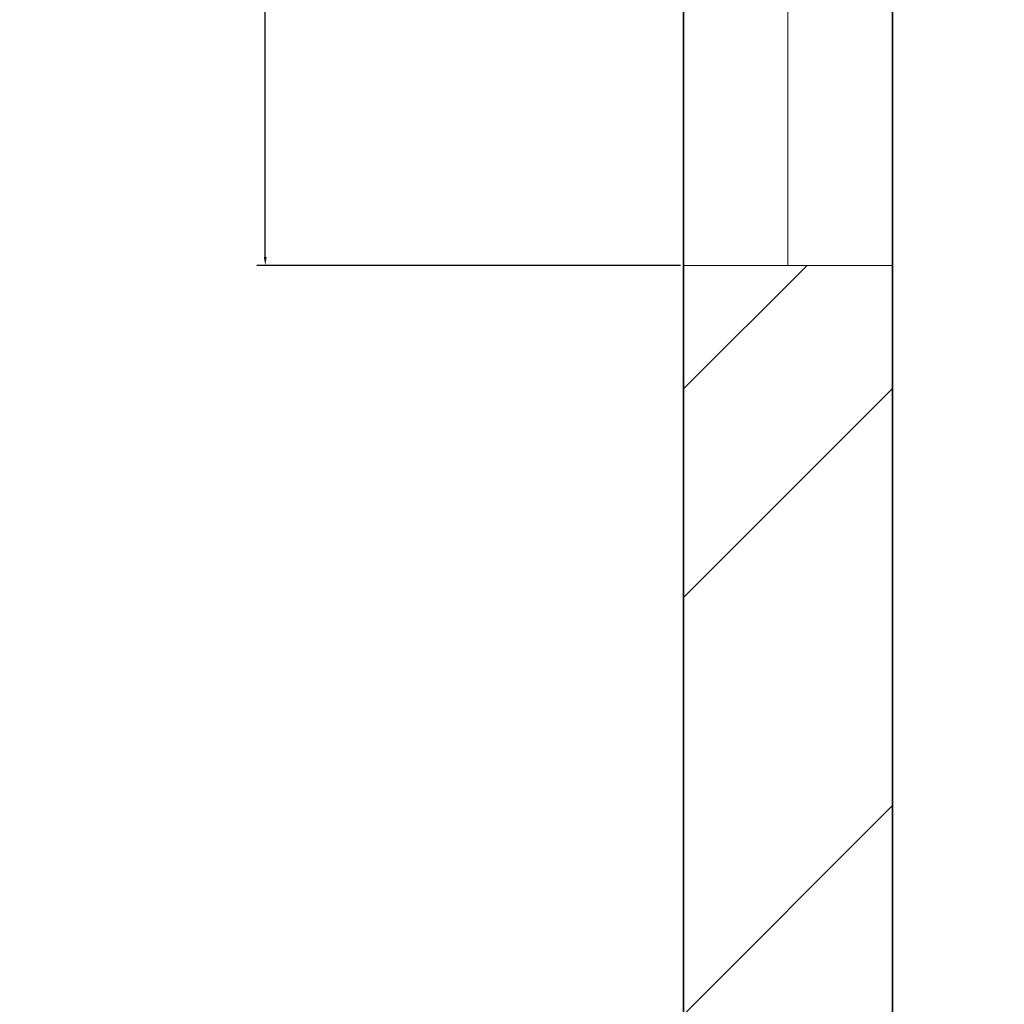
# Model space of a CAD drawing. Units: inches. Extents: x 1962 to 2771, y 1245 to 2660.
# Tile 23 of 114: x 2072 to 2093, y 1831 to 1852. Entities that reach past the tile are written whole.
import ezdxf

# ---------------------------------------------------------------- set-up
doc = ezdxf.new("R2010")
doc.units = ezdxf.units.IN
for name, color, linetype, lineweight in [('A-ANNO-DIMS', 2, 'Continuous', 18), ('A-GLAZ', 4, 'Continuous', 18), ('A-WALL', 7, 'Continuous', 35), ('A-WALL-PATT', 252, 'Continuous', 13)]:
    doc.layers.add(name, color=color, linetype=linetype, lineweight=lineweight)
doc.styles.get("Standard").update_dxf_attribs({"font": 'arial.ttf'})
doc.dimstyles.get("Standard").update_dxf_attribs({"dimtxt": 0.18, "dimasz": 0.18, "dimexe": 0.18, "dimexo": 0.0625, "dimgap": 0.09, "dimtad": 0, "dimtih": 1, "dimtoh": 1, "dimdec": 4, "dimzin": 0, "dimdsep": 46, "dimtxsty": 'Standard', "dimcen": 0.09, "dimadec": 0, "dimazin": 0, "dimtfac": 1, "dimtdec": 4, "dimtofl": 0, "dimtmove": 0, "dimatfit": 3, "dimfxl": 1, "dimtolj": 1, "dimtzin": 0, "dimarcsym": 0})

# ---------------------------------------------------------------- blocks, each defined once
blk = doc.blocks.new('WIN-60IN-A')
for p, q in [((2.25, 60), (2.25, 0)), ((2.25, 0), (0, 0)), ((0, 0), (4.5, 0))]:
    blk.add_line(p, q)
blk = doc.blocks.new('*D22')
at = {"layer": 'A-ANNO-DIMS', "color": 0, "lineweight": -2, "transparency": 16777216}
for p, q in [((2086.245, 1906.501), (2077.127, 1906.501)), ((2077.307, 1906.321), (2077.307, 1876.683)), ((2077.307, 1846.681), (2077.307, 1876.319)), ((2086.245, 1846.501), (2077.127, 1846.501))]:
    blk.add_line(p, q, dxfattribs=at)
at = {"layer": 'A-ANNO-DIMS', "color": 0, "transparency": 16777216}
for points in [[(2077.277, 1906.321), (2077.337, 1906.321), (2077.307, 1906.501)], [(2077.277, 1846.681), (2077.337, 1846.681), (2077.307, 1846.501)]]:
    blk.add_solid(points, dxfattribs=at)
at = {"layer": 'Defpoints', "color": 0, "transparency": 16777216}
for p in [(2077.307, 1906.501), (2086.307, 1906.501), (2086.307, 1846.501)]:
    blk.add_point(p, dxfattribs=at)
at = {"layer": 'A-ANNO-DIMS', "color": 0, "transparency": 16777216, "insert": (2077.307, 1876.501), "char_height": 0.18, "attachment_point": 5}
blk.add_mtext('\\A1;W3A 60 TYP.', dxfattribs=at)

msp = doc.modelspace()

# ---------------------------------------------------------------- hatches: boundary and pattern name
at = {"layer": 'A-WALL-PATT'}
h = msp.add_hatch(dxfattribs=at)
h.set_pattern_fill('ANSI32', color=256)
h.paths.add_polyline_path([(2090.8074, 2467.3437), (2141.6481, 2467.3437), (2141.6481, 2469.5937), (2141.6481, 2471.8437), (2086.3074, 2471.8437), (2086.3074, 2422.5333), (2090.8074, 2422.5333)])
h.paths.add_polyline_path([(2282.7664, 2471.8437), (2204.8982, 2471.8437), (2204.8982, 2467.3437), (2234.8074, 2467.3437), (2234.8074, 2311.3437), (2228.7492, 2311.3437), (2228.7492, 2306.8437), (2234.8074, 2306.8437), (2331.9227, 2306.8437), (2331.9227, 2309.0937), (2331.9227, 2311.3437), (2239.3074, 2311.3437), (2239.3074, 2467.3437), (2282.7664, 2467.3437), (2282.7664, 2469.5937)])
h.paths.add_polyline_path([(2471.4531, 2519.8437), (2552.011, 2519.8437), (2564.3996, 2519.8437), (2564.3996, 2511.1389), (2568.8996, 2511.1389), (2568.8996, 2524.3437), (2466.9531, 2524.3437), (2466.9531, 2471.8437), (2450.0749, 2471.8437), (2446.4672, 2471.8437), (2446.4672, 2467.3437), (2450.0749, 2467.3437), (2475.9988, 2467.3437), (2475.9988, 2469.5937), (2475.9988, 2471.8437), (2471.4531, 2471.8437)])
h.paths.add_polyline_path([(2575.2231, 2469.5937), (2575.2231, 2471.8437), (2568.8996, 2471.8437), (2568.8996, 2487.1389), (2564.3996, 2487.1389), (2564.3996, 2471.8437), (2556.511, 2471.8437), (2499.2904, 2471.8437), (2499.2904, 2467.3437), (2507.8074, 2467.3437), (2507.8074, 2311.3437), (2414.863, 2311.3437), (2414.863, 2306.8437), (2512.3074, 2306.8437), (2517.0114, 2306.8437), (2517.0114, 2309.0937), (2517.0114, 2311.3437), (2512.3074, 2311.3437), (2512.3074, 2467.3437), (2575.2231, 2467.3437)])
h.paths.add_polyline_path([(2660.8074, 2471.8437), (2600.9602, 2471.8437), (2600.9602, 2467.3437), (2656.3074, 2467.3437), (2656.3074, 2432.5704), (2660.8074, 2432.5704)])
h.paths.add_polyline_path([(2660.8074, 2372.5704), (2656.3074, 2372.5704), (2656.3074, 2311.3437), (2600.276, 2311.3437), (2600.276, 2309.0937), (2600.276, 2306.8437), (2656.3074, 2306.8437), (2656.3074, 2296.2593), (2660.8074, 2296.2593)])
h.paths.add_polyline_path([(2572.3074, 2306.8437), (2577.1385, 2306.8437), (2577.1385, 2311.3437), (2551.082, 2311.3437), (2551.082, 2306.8437), (2567.8074, 2306.8437), (2567.8074, 2258.8437), (2540.0574, 2258.8437), (2540.0574, 2256.5937), (2540.0574, 2254.3437), (2567.8074, 2254.3437), (2656.3074, 2254.3437), (2656.3074, 2236.9085), (2660.8074, 2236.9085), (2660.8074, 2272.2593), (2656.3074, 2272.2593), (2656.3074, 2258.8437), (2572.3074, 2258.8437)])
h.paths.add_polyline_path([(2512.3074, 2254.3437), (2518.8716, 2254.3437), (2518.8716, 2256.5937), (2518.8716, 2258.8437), (2507.8074, 2258.8437), (2507.8074, 2177.8437), (2567.8074, 2177.8437), (2567.8074, 2172.9628), (2572.3074, 2172.9628), (2572.3074, 2177.8437), (2656.3074, 2177.8437), (2656.3074, 2166.4846), (2660.8074, 2166.4846), (2660.8074, 2200.9085), (2656.3074, 2200.9085), (2656.3074, 2182.3437), (2512.3074, 2182.3437)])
h.paths.add_polyline_path([(2656.3074, 2129.8437), (2572.3074, 2129.8437), (2572.3074, 2150.3044), (2570.0574, 2150.3044), (2567.8074, 2150.3044), (2567.8074, 2129.8437), (2507.8074, 2129.8437), (2507.8074, 2116.3027), (2510.0574, 2116.3027), (2512.3074, 2116.3027), (2512.3074, 2125.3437), (2567.8074, 2125.3437), (2572.3074, 2125.3437), (2656.3074, 2125.3437)])
h.paths.add_polyline_path([(2090.8074, 2362.5333), (2086.3074, 2362.5333), (2086.3074, 2298.6242), (2090.8074, 2298.6242), (2090.8074, 2306.8437), (2174.8074, 2306.8437), (2174.8074, 2286.4178), (2179.3074, 2286.4178), (2179.3074, 2306.8437), (2192.8641, 2306.8437), (2192.8641, 2309.0937), (2192.8641, 2311.3437), (2090.8074, 2311.3437)])
h.paths.add_polyline_path([(2209.156, 2258.8437), (2179.3074, 2258.8437), (2179.3074, 2263.2236), (2177.0574, 2263.2236), (2174.8074, 2263.2236), (2174.8074, 2258.8437), (2090.8074, 2258.8437), (2090.8074, 2274.6242), (2086.3074, 2274.6242), (2086.3074, 2238.2967), (2088.5574, 2238.2967), (2090.8074, 2238.2967), (2090.8074, 2254.3437), (2209.156, 2254.3437)])
h.paths.add_polyline_path([(2090.8074, 2177.8437), (2234.8074, 2177.8437), (2234.8074, 2173.1428), (2239.3074, 2173.1428), (2239.3074, 2258.8437), (2230.8442, 2258.8437), (2230.8442, 2256.5937), (2230.8442, 2254.3437), (2234.8074, 2254.3437), (2234.8074, 2182.3437), (2090.8074, 2182.3437), (2090.8074, 2202.2967), (2086.3074, 2202.2967), (2086.3074, 2140.0389), (2090.8074, 2140.0389)])
h.paths.add_polyline_path([(2090.8074, 2080.0389), (2086.3074, 2080.0389), (2086.3074, 2033.8437), (2090.8074, 2033.8437)], flags=17)
h.paths.add_polyline_path([(2244.9405, 2033.8437), (2239.3074, 2033.8437), (2239.3074, 2142.0665), (2237.2592, 2142.0665), (2234.8074, 2142.0665), (2234.8074, 2033.8437), (2090.8074, 2033.8437), (2076.5204, 2033.8437), (2072.0204, 2033.8437), (2072.0204, 2000.4493), (2076.5204, 2000.4493), (2076.5204, 2029.3437), (2090.8074, 2029.3437), (2244.9405, 2029.3437), (2244.9405, 2031.5937)])
h.paths.add_polyline_path([(2234.8074, 1933.3437), (2076.5204, 1933.3437), (2076.5204, 1952.4493), (2074.2704, 1952.4493), (2072.0204, 1952.4493), (2072.0204, 1933.3437), (2072.0204, 1928.8437), (2234.8074, 1928.8437)])
h.paths.add_polyline_path([(2090.8074, 1928.8437), (2086.3074, 1928.8437), (2086.3074, 1906.5013), (2090.8074, 1906.5013)])
h.paths.add_polyline_path([(2090.8074, 1846.5013), (2086.3074, 1846.5013), (2086.3074, 1769.9917), (2088.5574, 1769.9917), (2090.8074, 1769.9917), (2090.8074, 1780.3437), (2234.8074, 1780.3437), (2234.8074, 1708.3437), (2230.3764, 1708.3437), (2230.3764, 1703.8437), (2239.3074, 1703.8437), (2239.3074, 1792.6669), (2237.0574, 1792.6669), (2234.8074, 1792.6669), (2234.8074, 1784.8437), (2090.8074, 1784.8437)])
h.paths.add_polyline_path([(2239.3074, 1928.8437), (2244.9405, 1928.8437), (2244.9405, 1931.0937), (2244.9405, 1933.3437), (2234.8074, 1933.3437), (2234.8074, 1928.8437), (2234.8074, 1825.5949), (2239.3074, 1825.5949)])
h.paths.add_polyline_path([(2148.0425, 1649.0937), (2148.0425, 1651.3437), (2090.8074, 1651.3437), (2090.8074, 1646.8437), (2148.0425, 1646.8437)], flags=0)
h.paths.add_polyline_path([(2207.5601, 1708.3437), (2090.8074, 1708.3437), (2090.8074, 1703.8437), (2174.8074, 1703.8437), (2174.8074, 1651.3437), (2170.4457, 1651.3437), (2170.4457, 1646.8437), (2195.9924, 1646.8437), (2195.9924, 1649.0937), (2195.9924, 1651.3437), (2179.3074, 1651.3437), (2179.3074, 1703.8437), (2207.5601, 1703.8437), (2207.5601, 1706.0937)])
h.paths.add_polyline_path([(2090.8074, 1733.9917), (2086.3074, 1733.9917), (2086.3074, 1696.1032), (2088.5574, 1696.1032), (2090.8074, 1696.1032)])
h.paths.add_polyline_path([(2090.8074, 1672.1032), (2086.3074, 1672.1032), (2086.3074, 1600.3335), (2090.8074, 1600.3335)])
h.paths.add_polyline_path([(2090.8074, 1540.3335), (2086.3074, 1540.3335), (2086.3074, 1486.3437), (2139.6766, 1486.3437), (2139.6766, 1490.8437), (2090.8074, 1490.8437)])
h.paths.add_polyline_path([(2302.3876, 1490.8437), (2239.3074, 1490.8437), (2239.3074, 1646.8437), (2335.9994, 1646.8437), (2335.9994, 1651.3437), (2229.884, 1651.3437), (2229.884, 1646.8437), (2234.8074, 1646.8437), (2234.8074, 1490.8437), (2202.7103, 1490.8437), (2202.7103, 1488.5937), (2202.7103, 1486.3437), (2275.0699, 1486.3437), (2275.0699, 1475.772), (2279.5699, 1475.772), (2279.5699, 1486.3437), (2302.3876, 1486.3437)])
h.paths.add_polyline_path([(2279.5699, 1451.772), (2275.0699, 1451.772), (2275.0699, 1438.3437), (2174.8074, 1438.3437), (2174.8074, 1486.3437), (2179.7922, 1486.3437), (2179.7922, 1490.8437), (2163.3585, 1490.8437), (2163.3585, 1488.5937), (2163.3585, 1486.3437), (2170.3074, 1486.3437), (2170.3074, 1433.8437), (2279.5699, 1433.8437)])
h.paths.add_polyline_path([(2427.2363, 1490.8437), (2375.8074, 1490.8437), (2375.8074, 1646.8437), (2381.6401, 1646.8437), (2381.6401, 1651.3437), (2365.887, 1651.3437), (2365.887, 1649.0937), (2365.887, 1646.8437), (2371.3074, 1646.8437), (2371.3074, 1490.8437), (2327.5627, 1490.8437), (2327.5627, 1488.5937), (2327.5627, 1486.3437), (2371.3074, 1486.3437), (2371.3074, 1433.8437), (2375.8074, 1433.8437), (2375.8074, 1486.3437), (2427.2363, 1486.3437)])
h.paths.add_polyline_path([(2512.3074, 1646.8437), (2519.4351, 1646.8437), (2519.4351, 1649.0937), (2519.4351, 1651.3437), (2507.8074, 1651.3437), (2416.0063, 1651.3437), (2416.0063, 1649.0937), (2416.0063, 1646.8437), (2507.8074, 1646.8437), (2507.8074, 1490.8437), (2497.0532, 1490.8437), (2497.0532, 1488.5937), (2497.0532, 1486.3437), (2574.9344, 1486.3437), (2574.9344, 1476.0181), (2579.4344, 1476.0181), (2579.4344, 1486.3437), (2584.4872, 1486.3437), (2584.3074, 1490.8437), (2512.3074, 1490.8437)])
h.paths.add_polyline_path([(2470.5091, 1486.3437), (2473.9767, 1486.3437), (2473.9767, 1490.8437), (2449.6605, 1490.8437), (2449.6605, 1488.5937), (2449.6605, 1486.3437), (2466.0091, 1486.3437), (2466.0091, 1433.8437), (2470.5091, 1433.8437), (2579.4344, 1433.8437), (2579.4344, 1452.0181), (2574.9344, 1452.0181), (2574.9344, 1438.3437), (2554.5091, 1438.3437), (2470.5091, 1438.3437)])
h.paths.add_polyline_path([(2656.3074, 1490.8437), (2611.86, 1490.8437), (2611.86, 1486.3437), (2656.3074, 1486.3437)])
h.paths.add_polyline_path([(2660.8074, 1532.7007), (2658.5574, 1532.7007), (2656.3074, 1532.7007), (2656.3074, 1486.3437), (2660.8074, 1486.3437)])
h.paths.add_polyline_path([(2660.8074, 1664.9663), (2656.3074, 1664.9663), (2656.3074, 1651.3437), (2602.2313, 1651.3437), (2602.2313, 1646.8437), (2656.3074, 1646.8437), (2656.3074, 1592.7007), (2660.8074, 1592.7007)])
h.paths.add_polyline_path([(2660.8074, 1724.5221), (2656.3074, 1724.5221), (2656.3074, 1703.8437), (2542.4725, 1703.8437), (2542.4725, 1699.3437), (2567.8074, 1699.3437), (2567.8074, 1651.3437), (2552.7766, 1651.3437), (2552.7766, 1649.0937), (2552.7766, 1646.8437), (2577.2878, 1646.8437), (2577.2878, 1649.0937), (2577.2878, 1651.3437), (2572.3074, 1651.3437), (2572.3074, 1699.3437), (2656.3074, 1699.3437), (2656.3074, 1688.9663), (2660.8074, 1688.9663)])
h.paths.add_polyline_path([(2660.8074, 1880.6524), (2656.3074, 1880.6524), (2656.3074, 1832.8437), (2512.3074, 1832.8437), (2512.3074, 1837.8959), (2507.8074, 1837.8959), (2507.8074, 1828.3437), (2567.8074, 1828.3437), (2567.8074, 1804.3437), (2572.3074, 1804.3437), (2572.3074, 1828.3437), (2656.3074, 1828.3437), (2656.3074, 1818.6778), (2660.8074, 1818.6778)])
h.paths.add_polyline_path([(2660.8074, 1794.6778), (2656.3074, 1794.6778), (2656.3074, 1780.3437), (2572.3074, 1780.3437), (2572.3074, 1783.0303), (2570.0574, 1783.0303), (2567.8074, 1783.0303), (2567.8074, 1780.3437), (2507.8074, 1780.3437), (2507.8074, 1699.3437), (2517.8858, 1699.3437), (2517.8858, 1701.5937), (2517.8858, 1703.8437), (2512.3074, 1703.8437), (2512.3074, 1775.8437), (2656.3074, 1775.8437), (2656.3074, 1760.5221), (2660.8074, 1760.5221)])
h.paths.add_polyline_path([(2660.8074, 1981.3437), (2660.8074, 2020.2808), (2658.5574, 2020.2808), (2656.3074, 2020.2808), (2656.3074, 1981.3437), (2512.3074, 1981.3437), (2512.3074, 2086.6996), (2507.8074, 2086.6996), (2507.8074, 1981.3437), (2375.8074, 1981.3437), (2375.8074, 1986.8505), (2373.5574, 1986.8505), (2371.3074, 1986.8505), (2371.3074, 1973.2607), (2375.8074, 1973.2607), (2375.8074, 1976.8437), (2507.8074, 1976.8437), (2507.8074, 1865.4281), (2510.0574, 1865.4281), (2512.3074, 1865.4281), (2512.3074, 1976.8437), (2660.8074, 1976.8437)])
h.paths.add_polyline_path([(2375.8074, 1940.297), (2373.5574, 1940.297), (2371.3074, 1940.297), (2371.3074, 1933.3437), (2278.4434, 1933.3437), (2278.4434, 1928.8437), (2371.3074, 1928.8437), (2371.3074, 1651.3437), (2375.8074, 1651.3437)])
h.paths.add_polyline_path([(2660.8074, 1976.8437), (2656.3074, 1976.8437), (2656.3074, 1940.6524), (2660.8074, 1940.6524)], flags=17)
h.paths.add_polyline_path([(2660.8074, 2142.4846), (2656.3074, 2142.4846), (2656.3074, 2080.2808), (2660.8074, 2080.2808)])
h.paths.add_polyline_path([(2381.4189, 2311.3437), (2375.8074, 2311.3437), (2375.8074, 2467.3437), (2424.7242, 2467.3437), (2424.7242, 2469.5937), (2424.7242, 2471.8437), (2375.8074, 2471.8437), (2375.8074, 2524.3437), (2371.3074, 2524.3437), (2371.3074, 2471.8437), (2307.2097, 2471.8437), (2307.2097, 2467.3437), (2371.3074, 2467.3437), (2371.3074, 2311.3437), (2366.8901, 2311.3437), (2366.8901, 2306.8437), (2371.3074, 2306.8437), (2371.3074, 2033.8437), (2279.6589, 2033.8437), (2279.6589, 2029.3437), (2371.3074, 2029.3437), (2371.3074, 2014.2598), (2375.8074, 2014.2598), (2375.8074, 2306.8437), (2381.4189, 2306.8437)])
h.paths.add_polyline_path([(2263.3074, 2524.3437), (2170.3074, 2524.3437), (2170.3074, 2519.8437), (2170.3074, 2471.8437), (2165.0312, 2471.8437), (2165.0312, 2467.3437), (2179.6721, 2467.3437), (2179.6721, 2469.5161), (2179.6721, 2471.8437), (2174.8074, 2471.8437), (2174.8074, 2519.8437), (2258.8074, 2519.8437), (2258.8074, 2511.6436), (2263.3074, 2511.6436)])
h.paths.add_polyline_path([(2245.0232, 1361.4123), (2492.9468, 1361.4123), (2492.9468, 1398.505), (2245.0232, 1398.505)], flags=9)
h.paths.add_polyline_path([(2388.1434, 2086.6936), (2425.0704, 2086.6936), (2425.0704, 2105.3509), (2388.1434, 2105.3509)], flags=9)
h.paths.add_polyline_path([(2404.922, 2242.6744), (2445.7337, 2242.6744), (2445.7337, 2261.3318), (2404.922, 2261.3318)], flags=9)
h.paths.add_polyline_path([(2269.4107, 2156.7935), (2306.3378, 2156.7935), (2306.3378, 2175.4508), (2269.4107, 2175.4508)], flags=9)
h.paths.add_polyline_path([(2269.3277, 2233.4343), (2306.2547, 2233.4343), (2306.2547, 2252.0917), (2269.3277, 2252.0917)], flags=9)
h.paths.add_polyline_path([(2431.6052, 2320.6922), (2470.4456, 2320.6922), (2470.4456, 2339.3495), (2431.6052, 2339.3495)], flags=25)
h.paths.add_polyline_path([(2249.6902, 2315.7608), (2288.5306, 2315.7608), (2288.5306, 2334.4182), (2249.6902, 2334.4182)], flags=25)
h.paths.add_polyline_path([(2096.9301, 2314.3181), (2135.7704, 2314.3181), (2135.7704, 2332.9755), (2096.9301, 2332.9755)], flags=25)
h.paths.add_polyline_path([(2134.3475, 2285.7089), (2161.4655, 2285.7089), (2161.4655, 2304.3662), (2134.3475, 2304.3662)], flags=9)
h.paths.add_polyline_path([(2126.5155, 2209.4076), (2159.9227, 2209.4076), (2159.9227, 2228.065), (2126.5155, 2228.065)], flags=25)
h.paths.add_polyline_path([(2110.5753, 2141.5299), (2149.4157, 2141.5299), (2149.4157, 2160.1872), (2110.5753, 2160.1872)], flags=25)
h.paths.add_polyline_path([(2249.8618, 1968.3317), (2286.3966, 1968.3317), (2286.3966, 1986.989), (2249.8618, 1986.989)], flags=9)
h.paths.add_polyline_path([(2395.9507, 1777.0051), (2436.7624, 1777.0051), (2436.7624, 1795.6625), (2395.9507, 1795.6625)], flags=9)
h.paths.add_polyline_path([(2398.5259, 1888.5651), (2435.0062, 1888.5651), (2435.0062, 1907.2224), (2398.5259, 1907.2224)], flags=25)
h.paths.add_polyline_path([(2259.3506, 1728.3559), (2296.2776, 1728.3559), (2296.2776, 1747.0132), (2259.3506, 1747.0132)], flags=9)
h.paths.add_polyline_path([(2271.3698, 1845.268), (2308.2968, 1845.268), (2308.2968, 1863.9253), (2271.3698, 1863.9253)], flags=9)
h.paths.add_polyline_path([(2120.9355, 1786.3027), (2159.7759, 1786.3027), (2159.7759, 1804.9601), (2120.9355, 1804.9601)], flags=25)
h.paths.add_polyline_path([(2121.3164, 1732.1043), (2154.7236, 1732.1043), (2154.7236, 1750.7616), (2121.3164, 1750.7616)], flags=25)
h.paths.add_polyline_path([(2118.3706, 1678.8997), (2147.5282, 1678.8997), (2147.5282, 1697.557), (2118.3706, 1697.557)], flags=25)
h.paths.add_polyline_path([(2385.9227, 1493.557), (2424.763, 1493.557), (2424.763, 1512.2143), (2385.9227, 1512.2143)], flags=25)
h.paths.add_polyline_path([(2248.7058, 1500.0256), (2287.5462, 1500.0256), (2287.5462, 1518.6829), (2248.7058, 1518.6829)], flags=25)
h.paths.add_polyline_path([(2104.1669, 1617.3771), (2143.0073, 1617.3771), (2143.0073, 1636.0344), (2104.1669, 1636.0344)], flags=9)
h.paths.add_polyline_path([(2096.0714, 1447.8824), (2137.3845, 1447.8824), (2137.3845, 1458.1859), (2096.0714, 1458.1859)], flags=9)
h.paths.add_polyline_path([(2180.6114, 1440.325), (2209.7689, 1440.325), (2209.7689, 1458.9823), (2180.6114, 1458.9823)], flags=25)
h.paths.add_polyline_path([(2316.1698, 1447.9637), (2357.4829, 1447.9637), (2357.4829, 1458.2673), (2316.1698, 1458.2673)], flags=9)
h.paths.add_polyline_path([(2397.6187, 1447.9637), (2438.9318, 1447.9637), (2438.9318, 1458.2673), (2397.6187, 1458.2673)], flags=9)
h.paths.add_polyline_path([(2473.0778, 1439.5953), (2502.2354, 1439.5953), (2502.2354, 1458.2527), (2473.0778, 1458.2527)], flags=25)
h.paths.add_polyline_path([(2589.7027, 1447.8819), (2631.0158, 1447.8819), (2631.0158, 1458.1855), (2589.7027, 1458.1855)], flags=9)
h.paths.add_polyline_path([(2522.4009, 1497.5285), (2561.2413, 1497.5285), (2561.2413, 1516.1859), (2522.4009, 1516.1859)], flags=25)
h.paths.add_polyline_path([(2579.6565, 1671.3482), (2608.8141, 1671.3482), (2608.8141, 1690.0056), (2579.6565, 1690.0056)], flags=25)
h.paths.add_polyline_path([(2544.7038, 1725.5064), (2578.1111, 1725.5064), (2578.1111, 1744.1637), (2544.7038, 1744.1637)], flags=25)
h.paths.add_polyline_path([(2578.1191, 1807.472), (2607.2766, 1807.472), (2607.2766, 1826.1293), (2578.1191, 1826.1293)], flags=25)
h.paths.add_polyline_path([(2595.0614, 1835.1839), (2633.9018, 1835.1839), (2633.9018, 1853.8413), (2595.0614, 1853.8413)], flags=25)
h.paths.add_polyline_path([(2567.0097, 2097.7035), (2605.8501, 2097.7035), (2605.8501, 2116.3609), (2567.0097, 2116.3609)], flags=9)
h.paths.add_polyline_path([(2586.644, 2134.6454), (2615.8015, 2134.6454), (2615.8015, 2153.3027), (2586.644, 2153.3027)], flags=9)
h.paths.add_polyline_path([(2544.6185, 2212.6783), (2578.0258, 2212.6783), (2578.0258, 2231.3356), (2544.6185, 2231.3356)], flags=25)
h.paths.add_polyline_path([(2577.0273, 2256.9023), (2606.1849, 2256.9023), (2606.1849, 2275.5597), (2577.0273, 2275.5597)], flags=24)
h.paths.add_polyline_path([(2605.2683, 2315.2821), (2644.1087, 2315.2821), (2644.1087, 2333.9395), (2605.2683, 2333.9395)], flags=25)
h.paths.add_polyline_path([(2583.1244, 2496.1815), (2624.4375, 2496.1815), (2624.4375, 2506.4851), (2583.1244, 2506.4851)], flags=9)
h.paths.add_polyline_path([(2474.761, 2497.0823), (2503.9185, 2497.0823), (2503.9185, 2515.7397), (2474.761, 2515.7397)], flags=25)
h.paths.add_polyline_path([(2387.5787, 2494.2563), (2428.902, 2494.2563), (2428.902, 2504.5598), (2387.5787, 2504.5598)], flags=9)
h.paths.add_polyline_path([(2300.1657, 2500.1564), (2341.4788, 2500.1564), (2341.4788, 2510.46), (2300.1657, 2510.46)], flags=25)
h.paths.add_polyline_path([(2176.8589, 2497.5843), (2206.0165, 2497.5843), (2206.0165, 2516.2416), (2176.8589, 2516.2416)], flags=25)
h.paths.add_polyline_path([(2097.4668, 2494.9762), (2138.7799, 2494.9762), (2138.7799, 2505.2798), (2097.4668, 2505.2798)], flags=9)

# ---------------------------------------------------------------- linework, layer by layer
at = {"layer": 'A-WALL'}
for p, q in [((2086.3074, 1928.8437), (2086.3074, 1486.3437)), ((2090.8074, 1928.8437), (2090.8074, 1784.8437))]:
    msp.add_line(p, q, dxfattribs=at)

# ---------------------------------------------------------------- block references
at = {"layer": 'A-GLAZ'}
msp.add_blockref('WIN-60IN-A', (2086.3074, 1846.5013), dxfattribs=at)

# ---------------------------------------------------------------- dimensions: what is measured, and where the dimension line sits
at = {"layer": 'A-ANNO-DIMS'}
dim = msp.add_linear_dim(base=(2077.3074, 1906.5013), p1=(2086.3074, 1846.5013), p2=(2086.3074, 1906.5013), angle=90, text='W3A <> TYP.', dimstyle='Standard', override={"dimdec": 0, "dimlfac": 1, "dimrnd": 0, "dimzin": 0, "dimdsep": 46, "dimlunit": 2}, dxfattribs=at)
dim.commit()
dim.dimension.update_dxf_attribs({"geometry": '*D22', "text_midpoint": (2077.3074, 1876.5013)})

doc.saveas('drawing.dxf')
